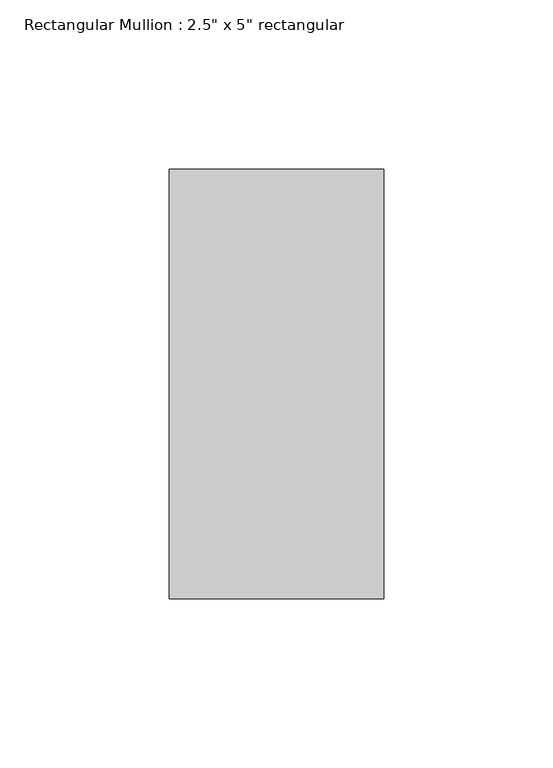
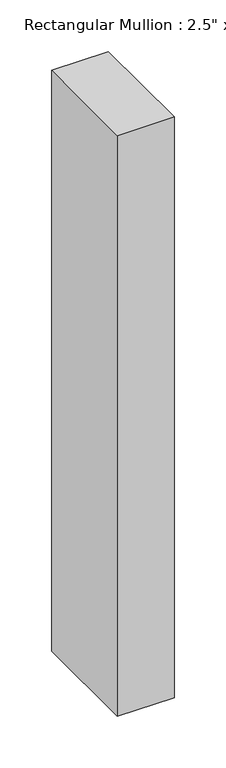
"""IFC4 building model written with IfcOpenShell, lengths in millimetres: member geometry."""

from ifc_helpers import new_model, si_unit, frame, origin, place, context, project, spatial, polyline, outline, extrude, source, transform, mapped, element, save


def member_f4ec938c(model_context):
    return source(origin(), model_context, "Body", "SweptSolid", [
        extrude(outline(polyline([(0.0, 63.5), (0.0, -63.5), (-63.5, -63.5), (-63.5, 63.5), (0.0, 63.5)])), frame((0.0, 0.0, -685.9455358), z_axis=(0.0, 0.0, 1.0), x_axis=(1.0, 0.0, 0.0)), (0.0, 0.0, 1.0), 685.9455358),
    ])


if __name__ == "__main__":
    model = new_model("IFC4")
    model_context = context("Model", 3, world=origin())
    ifc_project = project(units=[si_unit("LENGTHUNIT", "METRE", prefix="MILLI")], contexts=[model_context])
    site = spatial("IfcSite", under=ifc_project)
    building = spatial("IfcBuilding", under=site)
    placement = place(None, origin())
    member_shape = member_f4ec938c(model_context)
    element("IfcMember", 1, ObjectType="Rectangular Mullion : 2.5\" x 5\" rectangular", at=placement, inside=building, context=model_context, shape_type="MappedRepresentation", body=[
        mapped(member_shape, transform((0.0, 0.0, 0.0), x_axis=(1.0, 0.0, 0.0), y_axis=(0.0, 1.0, 0.0), z_axis=(0.0, 0.0, 1.0))),
    ])
    save(model, "model.ifc")

# Revit data of these elements
# Type "Rectangular Mullion : 2.5\" x 5\" rectangular"
#   built-in parameter 1007304 = 0.416667 (stored number, unit not read)
#   built-in parameter 1007301 = 0.104167 (stored number, unit not read)
#   built-in parameter 1007300 = 0.104167 (stored number, unit not read)
# Element 1 (IfcMember, "Rectangular Mullion : 2.5\" x 5\" rectangular")
#   Materials on its faces: "Aluminum"
# Materials
#   "Aluminum": class "Metal", colour RGB 247 247 247, transparency 0, Description = "Aluminum 6061", Cost = 0
